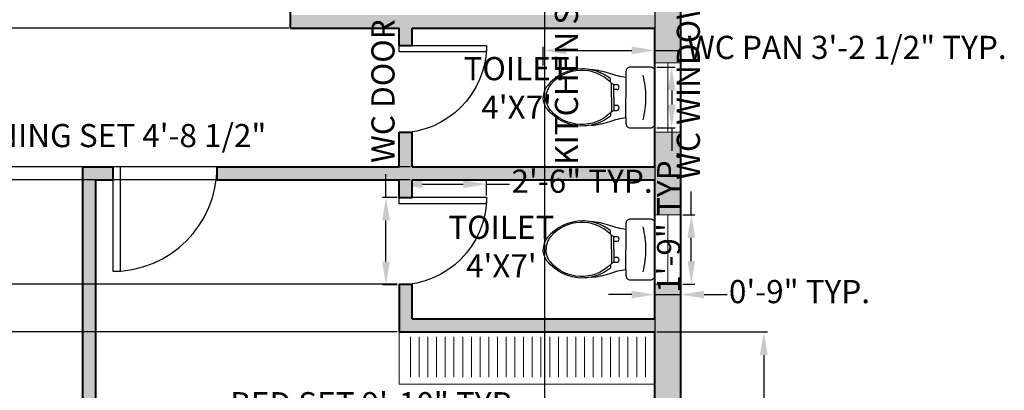
# Model space of a CAD drawing. Units: inches. Extents: x 2138 to 3265, y 2149 to 3392.
# Tile 5 of 13: x 2363 to 2703, y 2382 to 2511. Entities that reach past the tile are written whole.
import ezdxf

# ---------------------------------------------------------------- set-up
doc = ezdxf.new("R2010")
doc.units = ezdxf.units.IN
for name, color, linetype, lineweight in [('A-ANNO-DIMS', 2, 'Continuous', 18), ('A-AREA-IDEN', 7, 'Continuous', 18), ('A-DOOR', 22, 'Continuous', 25), ('A-FLOR-CASE', 30, 'Continuous', 20), ('A-FLOR-CASE-PATT', 251, 'Continuous', 13), ('A-FLOR-FIXT', 9, 'Continuous', 20), ('A-GLAZ', 150, 'Continuous', 18), ('A-WALL', 7, 'Continuous', 40), ('A-WALL-PATT', 142, 'Continuous', 13)]:
    doc.layers.add(name, color=color, linetype=linetype, lineweight=lineweight)
doc.layers.add('WC-Detail_dwgmodels.com', color=251, linetype='Continuous')
doc.layers.add('WC-Outline_dwgmodels.com', color=250, linetype='Continuous')
doc.styles.get("Standard").update_dxf_attribs({"font": 'arial.ttf'})
doc.dimstyles.new('ISO-25', dxfattribs={"dimtxt": 8, "dimasz": 8, "dimexe": 1.25, "dimexo": 0.625, "dimtad": 0, "dimdec": 1, "dimlunit": 4, "dimtxsty": 'Standard', "dimcen": 2.5, "dimadec": 0, "dimazin": 0, "dimtfac": 1, "dimtdec": 1, "dimtmove": 0, "dimatfit": 3, "dimfxl": 1, "dimarcsym": 0})

# ---------------------------------------------------------------- blocks, each defined once
blk = doc.blocks.new('pan')
at = {"layer": 'WC-Detail_dwgmodels.com'}
for p, q in [((2618, 2482.89), (2618, 2483.61)), ((2619.29, 2483.61), (2619.29, 2482.89)), ((2623.43, 2483.61), (2623.43, 2482.89)), ((2624.72, 2482.89), (2624.72, 2483.61)), ((2617.64, 2482.23), (2618, 2482.89)), ((2619.29, 2482.89), (2618, 2482.89)), ((2621.36, 2482.89), (2619.29, 2482.89)), ((2621.36, 2482.89), (2623.43, 2482.89)), ((2623.43, 2482.89), (2624.72, 2482.89)), ((2625.08, 2482.23), (2624.72, 2482.89))]:
    blk.add_line(p, q, dxfattribs=at)
for points in [[(2617.36, 2481.96, 0.434217), (2618, 2466.33, 0.182634), (2621.36, 2465.1, 2.693815)], [(2616.47, 2481.96, 0.094048), (2614.41, 2478.1, 0.16845)], [(2617.36, 2481.96), (2616.47, 2481.96, 0.416606)], [(2617.64, 2482.23, 0.008985), (2617.36, 2481.96, 0.182634)], [(2621.36, 2482.23), (2617.64, 2482.23, 0.008985)], [(2621.36, 2482.23), (2625.08, 2482.23, -0.444938)], [(2625.35, 2481.96, -0.434217), (2624.72, 2466.33, -0.182634), (2621.36, 2465.1, -2.693815)], [(2625.08, 2482.23, -0.008985), (2625.35, 2481.96, -0.182634)], [(2625.35, 2481.96), (2626.25, 2481.96, -0.416606)], [(2626.25, 2481.96, -0.105447), (2628.45, 2477.59, -0.16845)], [(2614.41, 2478.1, 0.026594), (2614.11, 2476.89, 0.16845)], [(2628.45, 2477.59, -0.015301), (2628.61, 2476.89, -0.16845)]]:
    blk.add_lwpolyline(points, format="xyb", dxfattribs=at)
for centre, radius, start, end in [((2621.37, 2468.01), 23.26, 90.028, 104.6712), ((2621.35, 2468.01), 23.26, 75.3288, 89.972), ((2618.64, 2483.61), 0.645, 0, 180), ((2624.07, 2483.61), 0.645, 0, 180)]:
    blk.add_arc(centre, radius, start, end, dxfattribs=at)
at = {"layer": 'WC-Outline_dwgmodels.com'}
for points in [[(2628.15, 2486.03, 0.414214), (2629.29, 2487.17), (2629.29, 2492.48, 0.414214), (2628.15, 2493.62), (2621.36, 2493.62), (2614.57, 2493.62, 0.414214), (2613.43, 2492.48), (2613.43, 2487.17, 0.414214), (2614.57, 2486.03), (2616.12, 2486.03, -0.052345), (2615.1, 2481.79, 0.071131), (2614.11, 2476.89, 0.160777)], [(2616.12, 2486.03), (2621.36, 2486.03, 0.414214)], [(2626.59, 2486.03), (2621.36, 2486.03, -0.414214)], [(2628.61, 2476.89, 0.071131), (2627.62, 2481.79, -0.052345), (2626.59, 2486.03), (2628.15, 2486.03, 0.414214)], [(2614.11, 2476.89, 0.048023), (2613.89, 2474.65, 0.16845)], [(2628.61, 2476.89, -0.048023), (2628.83, 2474.65, -0.16845)], [(2613.89, 2474.65, 0.230343), (2618.36, 2465.4, 0.16845), (2621.36, 2464.36, 2.883082)], [(2628.83, 2474.65, -0.230343), (2624.36, 2465.4, -0.16845), (2621.36, 2464.36, -2.883082)]]:
    blk.add_lwpolyline(points, format="xyb", dxfattribs=at)
blk = doc.blocks.new('door')
blk.add_lwpolyline([(2064.92, 2369.1), (2066.69, 2369.1), (2066.69, 2393.11), (2064.92, 2393.11)], close=True)
blk.add_arc((2066.69, 2369.1), 24.02, 90, 180)
blk = doc.blocks.new('GLAZ-SASH-24IN')
for p, q in [((0, 24), (9, 24)), ((4.5, 24), (4.5, 0)), ((0, 0), (9, 0))]:
    blk.add_line(p, q)
blk = doc.blocks.new('*D25')
at = {"layer": 'A-ANNO-DIMS', "color": 0, "lineweight": -2, "transparency": 16777216}
for p, q in [((2595.13, 2443.16), (2595.13, 2451.16)), ((2592.15, 2443.16), (2596.38, 2443.16)), ((2595.13, 2427.16), (2595.13, 2435.16)), ((2592.15, 2419.16), (2596.38, 2419.16))]:
    blk.add_line(p, q, dxfattribs=at)
at = {"layer": 'A-ANNO-DIMS', "color": 0, "transparency": 16777216}
for points in [[(2593.8, 2435.16), (2596.46, 2435.16), (2595.13, 2443.16)], [(2593.8, 2427.16), (2596.46, 2427.16), (2595.13, 2419.16)]]:
    blk.add_solid(points, dxfattribs=at)
at = {"layer": 'Defpoints', "color": 0, "transparency": 16777216}
for p in [(2591.53, 2443.16), (2595.13, 2443.16), (2591.53, 2419.16)]:
    blk.add_point(p, dxfattribs=at)
at = {"layer": 'A-ANNO-DIMS', "color": 0, "transparency": 16777216, "insert": (2595.13, 2513.27), "char_height": 8, "attachment_point": 5, "rotation": 90}
blk.add_mtext('WC WINDOW 2\'-0" TYP.', dxfattribs=at)
blk = doc.blocks.new('*D26')
at = {"layer": 'A-ANNO-DIMS', "color": 0, "lineweight": -2, "transparency": 16777216}
for p, q in [((2582.53, 2418.54), (2582.53, 2414.31)), ((2591.53, 2418.54), (2591.53, 2414.31)), ((2574.53, 2415.56), (2566.53, 2415.56)), ((2582.53, 2415.56), (2591.53, 2415.56)), ((2599.53, 2415.56), (2607.53, 2415.56))]:
    blk.add_line(p, q, dxfattribs=at)
at = {"layer": 'A-ANNO-DIMS', "color": 0, "transparency": 16777216}
for points in [[(2574.53, 2416.89), (2574.53, 2414.23), (2582.53, 2415.56)], [(2599.53, 2416.89), (2599.53, 2414.23), (2591.53, 2415.56)]]:
    blk.add_solid(points, dxfattribs=at)
at = {"layer": 'Defpoints', "color": 0, "transparency": 16777216}
for p in [(2582.53, 2419.16), (2591.53, 2419.16), (2591.53, 2415.56)]:
    blk.add_point(p, dxfattribs=at)
at = {"layer": 'A-ANNO-DIMS', "color": 0, "transparency": 16777216, "insert": (2632.54, 2415.56), "char_height": 8, "attachment_point": 5}
blk.add_mtext('0\'-9" TYP.', dxfattribs=at)
blk = doc.blocks.new('*D29')
at = {"layer": 'A-ANNO-DIMS', "color": 0, "lineweight": -2, "transparency": 16777216}
for p, q in [((2489.5, 2449.16), (2489.5, 2457.16)), ((2493.4, 2449.16), (2488.25, 2449.16)), ((2489.5, 2426.94), (2489.5, 2441.16)), ((2493.4, 2418.94), (2488.25, 2418.94))]:
    blk.add_line(p, q, dxfattribs=at)
at = {"layer": 'A-ANNO-DIMS', "color": 0, "transparency": 16777216}
for points in [[(2488.16, 2441.16), (2490.83, 2441.16), (2489.5, 2449.16)], [(2488.16, 2426.94), (2490.83, 2426.94), (2489.5, 2418.94)]]:
    blk.add_solid(points, dxfattribs=at)
at = {"layer": 'Defpoints', "color": 0, "transparency": 16777216}
for p in [(2489.5, 2449.16), (2494.03, 2449.16), (2494.03, 2418.94)]:
    blk.add_point(p, dxfattribs=at)
at = {"layer": 'A-ANNO-DIMS', "color": 0, "transparency": 16777216, "insert": (2489.5, 2511.51), "char_height": 8, "attachment_point": 5, "rotation": 90}
blk.add_mtext('WC DOOR 2\'-6" TYP.', dxfattribs=at)
blk = doc.blocks.new('*D30')
at = {"layer": 'A-ANNO-DIMS', "color": 0, "lineweight": -2, "transparency": 16777216}
for p, q in [((2494.03, 2449.79), (2494.03, 2454.95)), ((2502.03, 2453.7), (2516.26, 2453.7)), ((2524.26, 2449.79), (2524.26, 2454.95)), ((2524.26, 2453.7), (2532.26, 2453.7))]:
    blk.add_line(p, q, dxfattribs=at)
at = {"layer": 'A-ANNO-DIMS', "color": 0, "transparency": 16777216}
for points in [[(2502.03, 2455.03), (2502.03, 2452.36), (2494.03, 2453.7)], [(2516.26, 2455.03), (2516.26, 2452.36), (2524.26, 2453.7)]]:
    blk.add_solid(points, dxfattribs=at)
at = {"layer": 'Defpoints', "color": 0, "transparency": 16777216}
for p in [(2524.26, 2453.7), (2494.03, 2449.16), (2524.26, 2449.16)]:
    blk.add_point(p, dxfattribs=at)
at = {"layer": 'A-ANNO-DIMS', "color": 0, "transparency": 16777216, "insert": (2557.33, 2453.7), "char_height": 8, "attachment_point": 5}
blk.add_mtext('2\'-6" TYP.', dxfattribs=at)
blk = doc.blocks.new('*D33')
at = {"layer": 'A-ANNO-DIMS', "color": 0, "lineweight": -2, "transparency": 16777216}
for p, q in [((2543.88, 2494.76), (2543.88, 2501.18)), ((2582.53, 2494.76), (2582.53, 2501.18)), ((2551.88, 2499.93), (2574.53, 2499.93)), ((2582.53, 2499.93), (2590.53, 2499.93))]:
    blk.add_line(p, q, dxfattribs=at)
at = {"layer": 'A-ANNO-DIMS', "color": 0, "transparency": 16777216}
for points in [[(2551.88, 2501.26), (2551.88, 2498.6), (2543.88, 2499.93)], [(2574.53, 2501.26), (2574.53, 2498.6), (2582.53, 2499.93)]]:
    blk.add_solid(points, dxfattribs=at)
at = {"layer": 'Defpoints', "color": 0, "transparency": 16777216}
for p in [(2582.53, 2499.93), (2543.88, 2494.13), (2582.53, 2494.13)]:
    blk.add_point(p, dxfattribs=at)
at = {"layer": 'A-ANNO-DIMS', "color": 0, "transparency": 16777216, "insert": (2648.93, 2499.93), "char_height": 8, "attachment_point": 5}
blk.add_mtext('WC PAN 3\'-2 1/2" TYP.', dxfattribs=at)
blk = doc.blocks.new('*D34')
at = {"layer": 'A-ANNO-DIMS', "color": 0, "lineweight": -2, "transparency": 16777216}
for p, q in [((2583.15, 2494.13), (2589.58, 2494.13)), ((2588.33, 2486.13), (2588.33, 2481.19)), ((2583.15, 2473.19), (2589.58, 2473.19)), ((2588.33, 2473.19), (2588.33, 2465.19))]:
    blk.add_line(p, q, dxfattribs=at)
at = {"layer": 'A-ANNO-DIMS', "color": 0, "transparency": 16777216}
for points in [[(2586.99, 2486.13), (2589.66, 2486.13), (2588.33, 2494.13)], [(2586.99, 2481.19), (2589.66, 2481.19), (2588.33, 2473.19)]]:
    blk.add_solid(points, dxfattribs=at)
at = {"layer": 'Defpoints', "color": 0, "transparency": 16777216}
for p in [(2582.53, 2494.13), (2582.53, 2473.19), (2588.33, 2473.19)]:
    blk.add_point(p, dxfattribs=at)
at = {"layer": 'A-ANNO-DIMS', "color": 0, "transparency": 16777216, "insert": (2588.33, 2440.56), "char_height": 8, "attachment_point": 5, "rotation": 90}
blk.add_mtext('1\'-9" TYP.', dxfattribs=at)
blk = doc.blocks.new('*D35')
at = {"layer": 'A-ANNO-DIMS', "color": 0, "lineweight": -2, "transparency": 16777216}
for p, q in [((2426.72, 2359.73), (2426.72, 2378.07)), ((2544.83, 2359.73), (2544.83, 2378.07)), ((2418.72, 2376.82), (2410.72, 2376.82)), ((2426.72, 2376.82), (2432.38, 2376.82)), ((2544.83, 2376.82), (2539.18, 2376.82)), ((2552.83, 2376.82), (2560.83, 2376.82))]:
    blk.add_line(p, q, dxfattribs=at)
at = {"layer": 'A-ANNO-DIMS', "color": 0, "transparency": 16777216}
for points in [[(2418.72, 2378.16), (2418.72, 2375.49), (2426.72, 2376.82)], [(2552.83, 2378.16), (2552.83, 2375.49), (2544.83, 2376.82)]]:
    blk.add_solid(points, dxfattribs=at)
at = {"layer": 'Defpoints', "color": 0, "transparency": 16777216}
for p in [(2426.72, 2376.82), (2426.72, 2359.11), (2544.83, 2359.11)]:
    blk.add_point(p, dxfattribs=at)
at = {"layer": 'A-ANNO-DIMS', "color": 0, "transparency": 16777216, "insert": (2485.78, 2376.82), "char_height": 8, "attachment_point": 5}
blk.add_mtext('BED SET 9\'-10" TYP.', dxfattribs=at)
blk = doc.blocks.new('*D37')
at = {"layer": 'A-ANNO-DIMS', "color": 0, "lineweight": -2, "transparency": 16777216}
for p, q in [((2277.64, 2477.28), (2277.64, 2468.21)), ((2333.96, 2477.28), (2333.96, 2468.21)), ((2285.64, 2469.46), (2325.96, 2469.46)), ((2333.96, 2469.46), (2341.96, 2469.46))]:
    blk.add_line(p, q, dxfattribs=at)
at = {"layer": 'A-ANNO-DIMS', "color": 0, "transparency": 16777216}
for points in [[(2285.64, 2470.8), (2285.64, 2468.13), (2277.64, 2469.46)], [(2325.96, 2470.8), (2325.96, 2468.13), (2333.96, 2469.46)]]:
    blk.add_solid(points, dxfattribs=at)
at = {"layer": 'Defpoints', "color": 0, "transparency": 16777216}
for p in [(2277.64, 2477.91), (2333.96, 2477.91), (2333.96, 2469.46)]:
    blk.add_point(p, dxfattribs=at)
at = {"layer": 'A-ANNO-DIMS', "color": 0, "transparency": 16777216, "insert": (2395.87, 2469.46), "char_height": 8, "attachment_point": 5}
blk.add_mtext('DINING SET 4\'-8 1/2"', dxfattribs=at)
blk = doc.blocks.new('*D45')
at = {"layer": 'A-ANNO-DIMS', "color": 0, "lineweight": -2, "transparency": 16777216}
for p, q in [((2559, 2633.03), (2551.72, 2633.03)), ((2552.97, 2625.03), (2552.97, 2596.66)), ((2559, 2588.66), (2551.72, 2588.66)), ((2552.97, 2588.66), (2552.97, 2580.66))]:
    blk.add_line(p, q, dxfattribs=at)
at = {"layer": 'A-ANNO-DIMS', "color": 0, "transparency": 16777216}
for points in [[(2551.64, 2625.03), (2554.31, 2625.03), (2552.97, 2633.03)], [(2551.64, 2596.66), (2554.31, 2596.66), (2552.97, 2588.66)]]:
    blk.add_solid(points, dxfattribs=at)
at = {"layer": 'Defpoints', "color": 0, "transparency": 16777216}
for p in [(2559.63, 2633.03), (2552.97, 2588.66), (2559.63, 2588.66)]:
    blk.add_point(p, dxfattribs=at)
at = {"layer": 'A-ANNO-DIMS', "color": 0, "transparency": 16777216, "insert": (2552.97, 2519.59), "char_height": 8, "attachment_point": 5, "rotation": 90}
blk.add_mtext('KITCHEN SINK 3\'-8 1/2"', dxfattribs=at)
blk = doc.blocks.new('*D53')
at = {"layer": 'A-ANNO-DIMS', "color": 0, "lineweight": -2, "transparency": 16777216}
for p, q in [((2178.85, 2467.66), (2178.85, 2475.66)), ((2497.9, 2459.66), (2177.6, 2459.66)), ((2178.85, 2459.66), (2178.85, 2455.16)), ((2497.9, 2455.16), (2177.6, 2455.16)), ((2178.85, 2447.16), (2178.85, 2439.16))]:
    blk.add_line(p, q, dxfattribs=at)
at = {"layer": 'A-ANNO-DIMS', "color": 0, "transparency": 16777216}
for points in [[(2177.52, 2467.66), (2180.19, 2467.66), (2178.85, 2459.66)], [(2177.52, 2447.16), (2180.19, 2447.16), (2178.85, 2455.16)]]:
    blk.add_solid(points, dxfattribs=at)
at = {"layer": 'Defpoints', "color": 0, "transparency": 16777216}
for p in [(2498.53, 2459.66), (2178.85, 2455.16), (2498.53, 2455.16)]:
    blk.add_point(p, dxfattribs=at)
at = {"layer": 'A-ANNO-DIMS', "color": 0, "transparency": 16777216, "insert": (2178.85, 2418.58), "char_height": 8, "attachment_point": 5, "rotation": 90}
blk.add_mtext('0\'-4 1/2"', dxfattribs=at)
blk = doc.blocks.new('*D55')
at = {"layer": 'A-ANNO-DIMS', "color": 0, "lineweight": -2, "transparency": 16777216}
for p, q in [((2455.9, 2588.66), (2177.6, 2588.66)), ((2178.85, 2580.66), (2178.85, 2559.44)), ((2178.85, 2515.66), (2178.85, 2536.88)), ((2455.9, 2507.66), (2177.6, 2507.66))]:
    blk.add_line(p, q, dxfattribs=at)
at = {"layer": 'A-ANNO-DIMS', "color": 0, "transparency": 16777216}
for points in [[(2177.52, 2580.66), (2180.19, 2580.66), (2178.85, 2588.66)], [(2177.52, 2515.66), (2180.19, 2515.66), (2178.85, 2507.66)]]:
    blk.add_solid(points, dxfattribs=at)
at = {"layer": 'Defpoints', "color": 0, "transparency": 16777216}
for p in [(2456.53, 2588.66), (2178.85, 2507.66), (2456.53, 2507.66)]:
    blk.add_point(p, dxfattribs=at)
at = {"layer": 'A-ANNO-DIMS', "color": 0, "transparency": 16777216, "insert": (2178.85, 2548.16), "char_height": 8, "attachment_point": 5, "rotation": 90}
blk.add_mtext('6\'-9"', dxfattribs=at)
blk = doc.blocks.new('*D56')
at = {"layer": 'A-ANNO-DIMS', "color": 0, "lineweight": -2, "transparency": 16777216}
for p, q in [((2583.15, 2402.66), (2621.45, 2402.66)), ((2620.2, 2394.66), (2620.2, 2340.15)), ((2620.2, 2257.66), (2620.2, 2312.17)), ((2592.15, 2249.66), (2621.45, 2249.66))]:
    blk.add_line(p, q, dxfattribs=at)
at = {"layer": 'A-ANNO-DIMS', "color": 0, "transparency": 16777216}
for points in [[(2618.87, 2394.66), (2621.54, 2394.66), (2620.2, 2402.66)], [(2618.87, 2257.66), (2621.54, 2257.66), (2620.2, 2249.66)]]:
    blk.add_solid(points, dxfattribs=at)
at = {"layer": 'Defpoints', "color": 0, "transparency": 16777216}
for p in [(2582.53, 2402.66), (2620.2, 2402.66), (2591.53, 2249.66)]:
    blk.add_point(p, dxfattribs=at)
at = {"layer": 'A-ANNO-DIMS', "color": 0, "transparency": 16777216, "insert": (2620.2, 2326.16), "char_height": 8, "attachment_point": 5, "rotation": 90}
blk.add_mtext('12\'-9"', dxfattribs=at)
blk = doc.blocks.new('*D58')
at = {"layer": 'A-ANNO-DIMS', "color": 0, "lineweight": -2, "transparency": 16777216}
for p, q in [((2544.36, 2720.04), (2544.36, 2159.74)), ((2582.53, 2720.04), (2582.53, 2159.74)), ((2536.36, 2160.99), (2528.36, 2160.99)), ((2544.36, 2160.99), (2552.19, 2160.99)), ((2582.53, 2160.99), (2574.7, 2160.99)), ((2590.53, 2160.99), (2598.53, 2160.99))]:
    blk.add_line(p, q, dxfattribs=at)
at = {"layer": 'A-ANNO-DIMS', "color": 0, "transparency": 16777216}
for points in [[(2536.36, 2162.32), (2536.36, 2159.65), (2544.36, 2160.99)], [(2590.53, 2162.32), (2590.53, 2159.65), (2582.53, 2160.99)]]:
    blk.add_solid(points, dxfattribs=at)
at = {"layer": 'Defpoints', "color": 0, "transparency": 16777216}
for p in [(2544.36, 2720.66), (2582.53, 2720.66), (2544.36, 2160.99)]:
    blk.add_point(p, dxfattribs=at)
at = {"layer": 'A-ANNO-DIMS', "color": 0, "transparency": 16777216, "insert": (2563.45, 2160.99), "char_height": 8, "attachment_point": 5}
blk.add_mtext('3\'-2"', dxfattribs=at)
blk = doc.blocks.new('*D60')
at = {"layer": 'A-ANNO-DIMS', "color": 0, "lineweight": -2, "transparency": 16777216}
for p, q in [((2178.85, 2427.16), (2178.85, 2435.16)), ((2493.4, 2419.16), (2177.6, 2419.16)), ((2178.85, 2419.16), (2178.85, 2402.66)), ((2493.4, 2402.66), (2177.6, 2402.66)), ((2178.85, 2394.66), (2178.85, 2386.66))]:
    blk.add_line(p, q, dxfattribs=at)
at = {"layer": 'A-ANNO-DIMS', "color": 0, "transparency": 16777216}
for points in [[(2177.52, 2427.16), (2180.19, 2427.16), (2178.85, 2419.16)], [(2177.52, 2394.66), (2180.19, 2394.66), (2178.85, 2402.66)]]:
    blk.add_solid(points, dxfattribs=at)
at = {"layer": 'Defpoints', "color": 0, "transparency": 16777216}
for p in [(2494.03, 2419.16), (2178.85, 2402.66), (2494.03, 2402.66)]:
    blk.add_point(p, dxfattribs=at)
at = {"layer": 'A-ANNO-DIMS', "color": 0, "transparency": 16777216, "insert": (2178.85, 2366.46), "char_height": 8, "attachment_point": 5, "rotation": 90}
blk.add_mtext('1\'-4 1/2"', dxfattribs=at)

msp = doc.modelspace()

# ---------------------------------------------------------------- hatches: boundary and pattern name
at = {"layer": 'A-FLOR-CASE-PATT'}
h = msp.add_hatch(dxfattribs=at)
h.set_pattern_fill('ANSI31', color=256, scale=0.94791, angle=45, style=0)
h.paths.add_polyline_path([(2497.1, 2387.01), (2581.37, 2387.01), (2581.37, 2401.01), (2497.1, 2401.01)])
at = {"layer": 'A-WALL-PATT'}
h = msp.add_hatch(color=256, dxfattribs=at)
h.dxf.hatch_style = 1
h.paths.add_polyline_path([(2270.53, 2729.66), (2207.53, 2729.66), (2207.53, 2663.66), (2216.53, 2663.66), (2216.53, 2720.66), (2270.53, 2720.66)])
h.paths.add_polyline_path([(2484.36, 2729.66), (2330.53, 2729.66), (2330.53, 2720.66), (2384.53, 2720.66), (2384.53, 2546.66), (2372.53, 2546.66), (2372.53, 2542.16), (2389.03, 2542.16), (2389.03, 2720.66), (2484.36, 2720.66)])
h.paths.add_polyline_path([(2591.53, 2729.66), (2544.36, 2729.66), (2544.36, 2720.66), (2582.53, 2720.66), (2582.53, 2684.66), (2591.53, 2684.66)])
h.paths.add_polyline_path([(2591.53, 2624.66), (2582.53, 2624.66), (2582.53, 2588.66), (2456.53, 2588.66), (2456.53, 2584.16), (2582.53, 2584.16), (2582.53, 2512.16), (2456.53, 2512.16), (2456.53, 2507.66), (2494.03, 2507.66), (2494.03, 2501.66), (2498.53, 2501.66), (2498.53, 2507.66), (2582.53, 2507.66), (2582.53, 2495.66), (2591.53, 2495.66)])
h.paths.add_polyline_path([(2591.53, 2471.66), (2582.53, 2471.66), (2582.53, 2459.66), (2498.53, 2459.66), (2498.53, 2471.66), (2497.72, 2471.66, -0.030629), (2494.03, 2471.44), (2494.03, 2459.66), (2431.08, 2459.66, -0.013128), (2431.03, 2457.77), (2431.03, 2455.16), (2494.03, 2455.16), (2494.03, 2449.16), (2498.53, 2449.16), (2498.53, 2455.16), (2582.53, 2455.16), (2582.53, 2443.16), (2591.53, 2443.16)])
h.paths.add_polyline_path([(2591.53, 2419.16), (2582.53, 2419.16), (2582.53, 2407.16), (2498.53, 2407.16), (2498.53, 2419.16), (2497.72, 2419.16, -0.030629), (2494.03, 2418.94), (2494.03, 2402.66), (2582.53, 2402.66), (2582.53, 2360.66), (2591.53, 2360.66)])
h.paths.add_polyline_path([(2591.53, 2300.66), (2582.53, 2300.66), (2582.53, 2258.66), (2515.78, 2258.66), (2515.78, 2249.66), (2591.53, 2249.66)])
h.paths.add_polyline_path([(2455.78, 2258.66), (2389.03, 2258.66), (2389.03, 2455.16), (2395.03, 2455.16), (2395.03, 2459.66), (2384.53, 2459.66), (2384.53, 2258.66), (2375.53, 2258.66), (2375.53, 2249.66), (2455.78, 2249.66)])
h.paths.add_polyline_path([(2315.53, 2253.24), (2315.53, 2258.66), (2296.03, 2258.66), (2296.03, 2249.66), (2315.53, 2249.66)])
h.paths.add_polyline_path([(2236.03, 2258.66), (2216.53, 2258.66), (2216.53, 2290.16), (2207.53, 2290.16), (2207.53, 2249.66), (2236.03, 2249.66)])
h.paths.add_polyline_path([(2216.53, 2396.66), (2207.53, 2396.66), (2207.53, 2350.16), (2216.53, 2350.16)])
h.paths.add_polyline_path([(2216.53, 2603.66), (2207.53, 2603.66), (2207.53, 2456.66), (2216.53, 2456.66), (2216.53, 2542.16), (2264.53, 2542.16), (2264.53, 2470.16), (2252.53, 2470.16), (2252.53, 2465.66), (2269.03, 2465.66), (2269.03, 2542.16), (2336.48, 2542.16, -0.013128), (2336.53, 2544.05), (2336.53, 2546.66), (2216.53, 2546.66)])

# ---------------------------------------------------------------- linework, layer by layer
at = {"layer": 'A-FLOR-CASE'}
for q in [(2494.03, 2402.66), (2582.53, 2384.66)]:
    msp.add_line((2494.03, 2384.66), q, dxfattribs=at)
at = {"layer": 'A-GLAZ'}
for points in [[(2582.53, 2495.66), (2591.53, 2495.66), (2591.53, 2471.66), (2582.53, 2471.66)], [(2582.53, 2443.16), (2591.53, 2443.16), (2591.53, 2419.16), (2582.53, 2419.16)]]:
    msp.add_lwpolyline(points, close=True, dxfattribs=at)
at = {"layer": 'A-WALL'}
for p, q in [((2591.53, 2249.66), (2591.53, 2729.66)), ((2456.53, 2507.66), (2456.53, 2588.66)), ((2456.53, 2507.66), (2494.03, 2507.66)), ((2494.03, 2501.66), (2494.03, 2507.66)), ((2498.53, 2501.66), (2498.53, 2507.66)), ((2498.53, 2507.66), (2582.53, 2507.66)), ((2582.53, 2459.66), (2582.53, 2507.66)), ((2494.03, 2501.66), (2498.53, 2501.66)), ((2494.03, 2459.66), (2494.03, 2471.66)), ((2494.03, 2471.66), (2498.53, 2471.66)), ((2498.53, 2459.66), (2498.53, 2471.66)), ((2384.53, 2459.66), (2395.03, 2459.66)), ((2384.53, 2459.66), (2384.53, 2258.66)), ((2395.03, 2459.66), (2395.03, 2455.16)), ((2431.03, 2459.66), (2431.03, 2455.16)), ((2431.03, 2459.66), (2494.03, 2459.66)), ((2498.53, 2459.66), (2582.53, 2459.66)), ((2389.03, 2455.16), (2395.03, 2455.16)), ((2389.03, 2455.16), (2389.03, 2258.66)), ((2431.03, 2455.16), (2494.03, 2455.16)), ((2494.03, 2449.16), (2494.03, 2455.16)), ((2498.53, 2449.16), (2498.53, 2455.16)), ((2498.53, 2455.16), (2582.53, 2455.16)), ((2582.53, 2407.16), (2582.53, 2455.16)), ((2494.03, 2449.16), (2498.53, 2449.16)), ((2494.03, 2419.16), (2498.53, 2419.16)), ((2494.03, 2419.16), (2494.03, 2402.66)), ((2498.53, 2407.16), (2498.53, 2419.16)), ((2498.53, 2407.16), (2582.53, 2407.16)), ((2494.03, 2402.66), (2582.53, 2402.66)), ((2582.53, 2258.66), (2582.53, 2402.66))]:
    msp.add_line(p, q, dxfattribs=at)

# ---------------------------------------------------------------- block references
at = {"layer": 'A-DOOR'}
for p, xscale, yscale, zscale, rotation in [((-487.73, -99.49), -1.258608767172022, 1.258608767172022, 1.258608767172022, 270), ((5497.31, 6015.88), 1.501085369916538, 1.501085369916538, 1.501085369916538, 180), ((-487.73, -151.99), -1.258608767172022, 1.258608767172022, 1.258608767172022, 270)]:
    msp.add_blockref('door', p, dxfattribs=dict(at, xscale=xscale, yscale=yscale, zscale=zscale, rotation=rotation))
at = {"layer": 'A-FLOR-FIXT', "xscale": 1.320784017660098, "yscale": 1.320784017660098, "zscale": 1.320784017660098, "rotation": 270}
for p in [(-711, 5945.91), (-711, 5893.41)]:
    msp.add_blockref('pan', p, dxfattribs=at)
at = {"layer": 'A-GLAZ'}
for p in [(2582.53, 2471.66), (2582.53, 2419.16)]:
    msp.add_blockref('GLAZ-SASH-24IN', p, dxfattribs=at)

# ---------------------------------------------------------------- texts
at = {"layer": 'A-AREA-IDEN', "char_height": 8, "attachment_point": 1}
for insert in [(2507.63, 2497.63), (2502.35, 2442.81)]:
    msp.add_mtext_dynamic_manual_height_columns("\\pxqc;TOILET\\P4'X7'", width=54.1279, gutter_width=12.5, heights=[0], dxfattribs=dict(at, insert=insert))

# ---------------------------------------------------------------- dimensions: what is measured, and where the dimension line sits
at = {"layer": 'A-ANNO-DIMS'}
dim = msp.add_linear_dim(base=(2544.36, 2160.99), p1=(2582.53, 2720.66), p2=(2544.36, 2720.66), dimstyle='ISO-25', override={"dimdec": 1, "dimlfac": 1, "dimrnd": 0, "dimzin": 1, "dimdsep": 46, "dimlunit": 4, "dimfrac": 2}, dxfattribs=at)
dim.commit()
dim.dimension.update_dxf_attribs({"geometry": '*D58', "text_midpoint": (2563.45, 2160.99)})
for base, p1, p2, angle, text, picture, middle in [((2552.97, 2588.66), (2559.63, 2633.03), (2559.63, 2588.66), 270, 'KITCHEN SINK <>', '*D45', (2552.97, 2519.59)), ((2595.13, 2443.16), (2591.53, 2419.16), (2591.53, 2443.16), 90, 'WC WINDOW <> TYP.', '*D25', (2595.13, 2513.27)), ((2489.5, 2449.16), (2494.03, 2418.94), (2494.03, 2449.16), 90, 'WC DOOR <> TYP.', '*D29', (2489.5, 2511.51)), ((2588.33, 2473.19), (2582.53, 2494.13), (2582.53, 2473.19), 270, '<> TYP.', '*D34', (2588.33, 2440.56)), ((2426.72, 2376.82), (2544.83, 2359.11), (2426.72, 2359.11), 180, 'BED SET <> TYP.', '*D35', (2485.78, 2376.82))]:
    dim = msp.add_linear_dim(base=base, p1=p1, p2=p2, angle=angle, text=text, dimstyle='ISO-25', override={"dimdec": 1, "dimlfac": 1, "dimrnd": 0, "dimzin": 1, "dimdsep": 46, "dimlunit": 4, "dimfrac": 2}, dxfattribs=at)
    dim.commit()
    dim.dimension.update_dxf_attribs({"geometry": picture, "text_midpoint": middle})
for base, p1, p2, picture, middle in [((2178.85, 2507.66), (2456.53, 2588.66), (2456.53, 2507.66), '*D55', (2178.85, 2548.16)), ((2178.85, 2455.16), (2498.53, 2459.66), (2498.53, 2455.16), '*D53', (2178.85, 2418.58)), ((2178.85, 2402.66), (2494.03, 2419.16), (2494.03, 2402.66), '*D60', (2178.85, 2366.46)), ((2620.2, 2402.66), (2591.53, 2249.66), (2582.53, 2402.66), '*D56', (2620.2, 2326.16))]:
    dim = msp.add_linear_dim(base=base, p1=p1, p2=p2, angle=90, dimstyle='ISO-25', override={"dimdec": 1, "dimlfac": 1, "dimrnd": 0, "dimzin": 1, "dimdsep": 46, "dimlunit": 4, "dimfrac": 2}, dxfattribs=at)
    dim.commit()
    dim.dimension.update_dxf_attribs({"geometry": picture, "text_midpoint": middle})
for base, p1, p2, text, picture, middle in [((2582.5295, 2499.9306), (2543.8826, 2494.1336), (2582.5295, 2494.1336), 'WC PAN <> TYP.', '*D33', (2648.9253, 2499.9306)), ((2333.96, 2469.46), (2277.64, 2477.91), (2333.96, 2477.91), 'DINING SET <>', '*D37', (2395.87, 2469.46)), ((2524.26, 2453.7), (2494.03, 2449.16), (2524.26, 2449.16), '<> TYP.', '*D30', (2557.33, 2453.7)), ((2591.53, 2415.56), (2582.53, 2419.16), (2591.53, 2419.16), '<> TYP.', '*D26', (2632.54, 2415.56))]:
    dim = msp.add_linear_dim(base=base, p1=p1, p2=p2, text=text, dimstyle='ISO-25', override={"dimdec": 1, "dimlfac": 1, "dimrnd": 0, "dimzin": 1, "dimdsep": 46, "dimlunit": 4, "dimfrac": 2}, dxfattribs=at)
    dim.commit()
    dim.dimension.update_dxf_attribs({"geometry": picture, "text_midpoint": middle})

doc.saveas('drawing.dxf')
